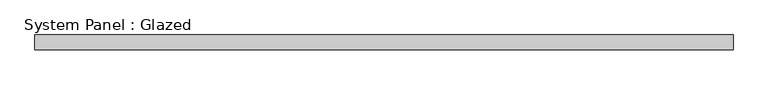
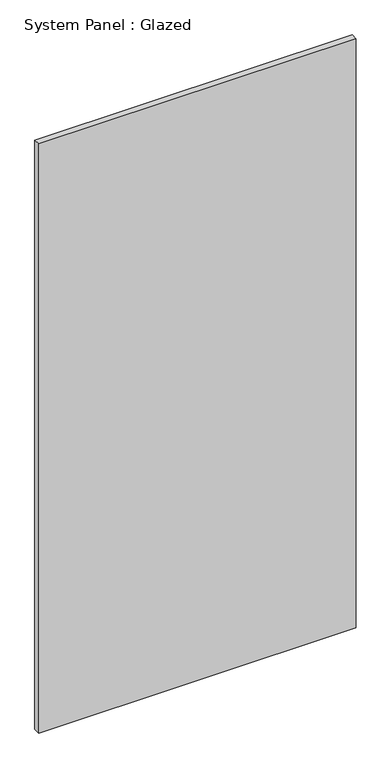
"""IFC4 building model written with IfcOpenShell, lengths in millimetres: plate geometry, System Panel : Glazed."""

from ifc_helpers import new_model, si_unit, origin, origin_with_axes, place, context, project, spatial, polyline, outline, extrude, source, transform, mapped, element, save


def system_panel_glazed_74eece19(model_context):
    return source(origin(), model_context, "Body", "SweptSolid", [
        extrude(outline(polyline([(597.5350001, 19.05), (-597.5350001, 19.05), (-597.5350001, 44.45), (597.5350001, 44.45), (597.5350001, 19.05)])), origin_with_axes(), (0.0, 0.0, 1.0), 2343.15),
    ])


if __name__ == "__main__":
    model = new_model("IFC4")
    model_context = context("Model", 3, world=origin())
    ifc_project = project(units=[si_unit("LENGTHUNIT", "METRE", prefix="MILLI")], contexts=[model_context])
    site = spatial("IfcSite", under=ifc_project)
    building = spatial("IfcBuilding", under=site)
    placement = place(None, origin())
    system_panel_glazed_shape = system_panel_glazed_74eece19(model_context)
    element("IfcPlate", 1, ObjectType="System Panel : Glazed", at=placement, inside=building, context=model_context, shape_type="MappedRepresentation", body=[
        mapped(system_panel_glazed_shape, transform((0.0, 0.0, 0.0), x_axis=(1.0, 0.0, 0.0), y_axis=(0.0, 1.0, 0.0), z_axis=(0.0, 0.0, 1.0))),
    ])
    save(model, "model.ifc")

# Revit data of these elements
# Type "System Panel : Glazed"
#   Construction Type Id = "GSP4R"
#   Analytic Construction = "1/8 in Pilkington single glazing"
#   Visual Light Transmittance = 0.9
#   Solar Heat Gain Coefficient = 0.86
#   Heat Transfer Coefficient (U) = 1.18115 BTU/(h·ft²·°F)
#   Define Thermal Properties by = 1
# Element 1 (IfcPlate, "System Panel : Glazed")
#   Materials on its faces: "Glass"
# Materials
#   "Glass": class "Glass", colour RGB 0 128 192, transparency 0.75, Description = "Soda Lime Glass", Cost = 0
